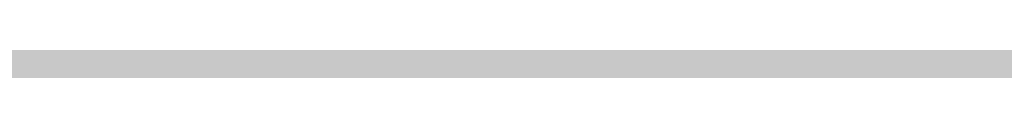
# Model space of a CAD drawing. Units: millimetres. Extents: x -22994 to 29398, y -19990 to 20176.
# Tile 97 of 135: x 229.428 to 230.597, y 84.571 to 84.585. Entities that reach past the tile are written whole.
import ezdxf
from ezdxf import colors
from ezdxf.entities.mleader import LeaderData, LeaderLine
from ezdxf.math import Vec2, Vec3

# ---------------------------------------------------------------- set-up
doc = ezdxf.new("R2010")
doc.units = ezdxf.units.MM
doc.header["$MEASUREMENT"] = 0
doc.layers.add('M-ANNO-TEXT', color=7, linetype='Continuous', lineweight=25)
doc.layers.add('M-DIMS', color=2, linetype='Continuous', lineweight=18)
doc.styles.get("Standard").update_dxf_attribs({"font": 'arial.ttf'})
doc.dimstyles.get("Standard").update_dxf_attribs({"dimtxt": 0.18, "dimasz": 10000, "dimexe": 0.18, "dimexo": 0.0625, "dimgap": 0.09, "dimtad": 0, "dimtih": 1, "dimtoh": 1, "dimdec": 0, "dimzin": 0, "dimdsep": 46, "dimtxsty": 'Standard', "dimcen": 0.09, "dimadec": 0, "dimazin": 0, "dimtfac": 1, "dimtdec": 0, "dimtofl": 0, "dimtmove": 0, "dimatfit": 3, "dimfxl": 1, "dimtolj": 1, "dimtzin": 0, "dimlwd": 30, "dimarcsym": 0})

# ---------------------------------------------------------------- blocks, each defined once
blk = doc.blocks.new('*D2')
at = {"layer": 'Defpoints', "color": 0, "transparency": 16777216}
for p in [(6.6773, 10.2713), (290.852, 10.2713), (290.852, -5.0787)]:
    blk.add_point(p, dxfattribs=at)
at = {"layer": 'M-DIMS', "color": 0, "lineweight": -2, "transparency": 16777216}
for p, q in [((6.6773, 10.2088), (6.6773, -5.2587)), ((290.852, 10.2088), (290.852, -5.2587))]:
    blk.add_line(p, q, dxfattribs=at)
at = {"layer": 'M-DIMS', "color": 0, "lineweight": 30, "transparency": 16777216}
for p, q in [((-9993.3227, -5.0787), (-19993.3227, -5.0787)), ((10290.852, -5.0787), (20290.852, -5.0787))]:
    blk.add_line(p, q, dxfattribs=at)
at = {"layer": 'M-DIMS', "color": 0, "transparency": 16777216}
for points in [[(-9993.3227, 1661.5879), (-9993.3227, -1671.7454), (6.6773, -5.0787)], [(10290.852, 1661.5879), (10290.852, -1671.7454), (290.852, -5.0787)]]:
    blk.add_solid(points, dxfattribs=at)
at = {"layer": 'M-DIMS', "color": 0, "transparency": 16777216, "insert": (148.7647, -5.0787), "char_height": 0.18, "attachment_point": 5}
blk.add_mtext('\\A1;284.2', dxfattribs=at)
blk = doc.blocks.new('*D3')
at = {"layer": 'Defpoints', "color": 0, "transparency": 16777216}
for p in [(110.2647, 204.1654), (110.2647, 176.3662), (95.8327, 127.967)]:
    blk.add_point(p, dxfattribs=at)
at = {"layer": 'M-DIMS', "color": 0, "lineweight": -2, "transparency": 16777216}
for p, q in [((95.8327, 128.0295), (95.8327, 204.3454)), ((110.2647, 176.4287), (110.2647, 204.3454))]:
    blk.add_line(p, q, dxfattribs=at)
at = {"layer": 'M-DIMS', "color": 0, "lineweight": 30, "transparency": 16777216}
for p, q in [((-9904.1673, 204.1654), (-19904.1673, 204.1654)), ((10110.2647, 204.1654), (20110.2647, 204.1654))]:
    blk.add_line(p, q, dxfattribs=at)
at = {"layer": 'M-DIMS', "color": 0, "transparency": 16777216}
for points in [[(-9904.1673, 1870.8321), (-9904.1673, -1462.5013), (95.8327, 204.1654)], [(10110.2647, 1870.8321), (10110.2647, -1462.5013), (110.2647, 204.1654)]]:
    blk.add_solid(points, dxfattribs=at)
at = {"layer": 'M-DIMS', "color": 0, "transparency": 16777216, "insert": (103.0487, 204.1654), "char_height": 0.18, "attachment_point": 5}
blk.add_mtext('\\A1;14.432', dxfattribs=at)
blk = doc.blocks.new('*D4')
at = {"layer": 'Defpoints', "color": 0, "transparency": 16777216}
for p in [(116.2647, 204.1654), (110.2647, 176.3662), (116.2647, 176.3662)]:
    blk.add_point(p, dxfattribs=at)
at = {"layer": 'M-DIMS', "color": 0, "lineweight": -2, "transparency": 16777216}
for p, q in [((110.2647, 176.4287), (110.2647, 204.3454)), ((116.2647, 176.4287), (116.2647, 204.3454))]:
    blk.add_line(p, q, dxfattribs=at)
at = {"layer": 'M-DIMS', "color": 0, "lineweight": 30, "transparency": 16777216}
for p, q in [((-9889.7353, 204.1654), (-19889.7353, 204.1654)), ((10116.2647, 204.1654), (20116.2647, 204.1654))]:
    blk.add_line(p, q, dxfattribs=at)
at = {"layer": 'M-DIMS', "color": 0, "transparency": 16777216}
for points in [[(-9889.7353, 1870.8321), (-9889.7353, -1462.5013), (110.2647, 204.1654)], [(10116.2647, 1870.8321), (10116.2647, -1462.5013), (116.2647, 204.1654)]]:
    blk.add_solid(points, dxfattribs=at)
at = {"layer": 'M-DIMS', "color": 0, "transparency": 16777216, "insert": (113.2647, 204.1654), "char_height": 0.18, "attachment_point": 5}
blk.add_mtext('\\A1;6', dxfattribs=at)
blk = doc.blocks.new('*D5')
at = {"layer": 'Defpoints', "color": 0, "transparency": 16777216}
for p in [(181.2647, 204.1654), (116.2647, 176.3662), (181.2647, 176.3662)]:
    blk.add_point(p, dxfattribs=at)
at = {"layer": 'M-DIMS', "color": 0, "lineweight": -2, "transparency": 16777216}
for p, q in [((116.2647, 176.4287), (116.2647, 204.3454)), ((181.2647, 176.4287), (181.2647, 204.3454))]:
    blk.add_line(p, q, dxfattribs=at)
at = {"layer": 'M-DIMS', "color": 0, "lineweight": 30, "transparency": 16777216}
for p, q in [((-9883.7353, 204.1654), (-19883.7353, 204.1654)), ((10181.2647, 204.1654), (20181.2647, 204.1654))]:
    blk.add_line(p, q, dxfattribs=at)
at = {"layer": 'M-DIMS', "color": 0, "transparency": 16777216}
for points in [[(-9883.7353, 1870.8321), (-9883.7353, -1462.5013), (116.2647, 204.1654)], [(10181.2647, 1870.8321), (10181.2647, -1462.5013), (181.2647, 204.1654)]]:
    blk.add_solid(points, dxfattribs=at)
at = {"layer": 'M-DIMS', "color": 0, "transparency": 16777216, "insert": (148.7647, 204.1654), "char_height": 0.18, "attachment_point": 5}
blk.add_mtext('\\A1;65', dxfattribs=at)
blk = doc.blocks.new('*D6')
at = {"layer": 'Defpoints', "color": 0, "transparency": 16777216}
for p in [(187.2647, 204.1654), (181.2647, 176.3662), (187.2647, 176.3662)]:
    blk.add_point(p, dxfattribs=at)
at = {"layer": 'M-DIMS', "color": 0, "lineweight": -2, "transparency": 16777216}
for p, q in [((181.2647, 176.4287), (181.2647, 204.3454)), ((187.2647, 176.4287), (187.2647, 204.3454))]:
    blk.add_line(p, q, dxfattribs=at)
at = {"layer": 'M-DIMS', "color": 0, "lineweight": 30, "transparency": 16777216}
for p, q in [((-9818.7353, 204.1654), (-19818.7353, 204.1654)), ((10187.2647, 204.1654), (20187.2647, 204.1654))]:
    blk.add_line(p, q, dxfattribs=at)
at = {"layer": 'M-DIMS', "color": 0, "transparency": 16777216}
for points in [[(-9818.7353, 1870.8321), (-9818.7353, -1462.5013), (181.2647, 204.1654)], [(10187.2647, 1870.8321), (10187.2647, -1462.5013), (187.2647, 204.1654)]]:
    blk.add_solid(points, dxfattribs=at)
at = {"layer": 'M-DIMS', "color": 0, "transparency": 16777216, "insert": (184.2647, 204.1654), "char_height": 0.18, "attachment_point": 5}
blk.add_mtext('\\A1;6', dxfattribs=at)
blk = doc.blocks.new('*D7')
at = {"layer": 'Defpoints', "color": 0, "transparency": 16777216}
for p in [(201.6967, 204.1654), (187.2647, 176.3662), (201.6967, 127.967)]:
    blk.add_point(p, dxfattribs=at)
at = {"layer": 'M-DIMS', "color": 0, "lineweight": -2, "transparency": 16777216}
for p, q in [((187.2647, 176.4287), (187.2647, 204.3454)), ((201.6967, 128.0295), (201.6967, 204.3454))]:
    blk.add_line(p, q, dxfattribs=at)
at = {"layer": 'M-DIMS', "color": 0, "lineweight": 30, "transparency": 16777216}
for p, q in [((-9812.7353, 204.1654), (-19812.7353, 204.1654)), ((10201.6967, 204.1654), (20201.6967, 204.1654))]:
    blk.add_line(p, q, dxfattribs=at)
at = {"layer": 'M-DIMS', "color": 0, "transparency": 16777216}
for points in [[(-9812.7353, 1870.8321), (-9812.7353, -1462.5013), (187.2647, 204.1654)], [(10201.6967, 1870.8321), (10201.6967, -1462.5013), (201.6967, 204.1654)]]:
    blk.add_solid(points, dxfattribs=at)
at = {"layer": 'M-DIMS', "color": 0, "transparency": 16777216, "insert": (194.4807, 204.1654), "char_height": 0.18, "attachment_point": 5}
blk.add_mtext('\\A1;14.432', dxfattribs=at)
blk = doc.blocks.new('*D8')
at = {"layer": 'Defpoints', "color": 0, "transparency": 16777216}
for p in [(227.6485, 204.1654), (227.6485, 146.7296), (201.6967, 127.967)]:
    blk.add_point(p, dxfattribs=at)
at = {"layer": 'M-DIMS', "color": 0, "lineweight": -2, "transparency": 16777216}
for p, q in [((201.6967, 128.0295), (201.6967, 204.3454)), ((227.6485, 146.7921), (227.6485, 204.3454))]:
    blk.add_line(p, q, dxfattribs=at)
at = {"layer": 'M-DIMS', "color": 0, "lineweight": 30, "transparency": 16777216}
for p, q in [((-9798.3033, 204.1654), (-19798.3033, 204.1654)), ((10227.6485, 204.1654), (20227.6485, 204.1654))]:
    blk.add_line(p, q, dxfattribs=at)
at = {"layer": 'M-DIMS', "color": 0, "transparency": 16777216}
for points in [[(-9798.3033, 1870.8321), (-9798.3033, -1462.5013), (201.6967, 204.1654)], [(10227.6485, 1870.8321), (10227.6485, -1462.5013), (227.6485, 204.1654)]]:
    blk.add_solid(points, dxfattribs=at)
at = {"layer": 'M-DIMS', "color": 0, "transparency": 16777216, "insert": (214.6726, 204.1654), "char_height": 0.18, "attachment_point": 5}
blk.add_mtext('\\A1;25.95', dxfattribs=at)
blk = doc.blocks.new('*D9')
at = {"layer": 'Defpoints', "color": 0, "transparency": 16777216}
for p in [(187.2647, 176.3662), (306.202, 176.3662), (290.852, 10.2713)]:
    blk.add_point(p, dxfattribs=at)
at = {"layer": 'M-DIMS', "color": 0, "lineweight": 30, "transparency": 16777216}
for p, q in [((306.202, 10176.3662), (306.202, 20176.3662)), ((306.202, -9989.7287), (306.202, -19989.7287))]:
    blk.add_line(p, q, dxfattribs=at)
at = {"layer": 'M-DIMS', "color": 0, "lineweight": -2, "transparency": 16777216}
for p, q in [((187.3272, 176.3662), (306.382, 176.3662)), ((290.9145, 10.2713), (306.382, 10.2713))]:
    blk.add_line(p, q, dxfattribs=at)
at = {"layer": 'M-DIMS', "color": 0, "transparency": 16777216}
for points in [[(-1360.4646, 10176.3662), (1972.8687, 10176.3662), (306.202, 176.3662)], [(-1360.4646, -9989.7287), (1972.8687, -9989.7287), (306.202, 10.2713)]]:
    blk.add_solid(points, dxfattribs=at)
at = {"layer": 'M-DIMS', "color": 0, "transparency": 16777216, "insert": (306.202, 93.3187), "char_height": 0.18, "attachment_point": 5}
blk.add_mtext('\\A1;166.1', dxfattribs=at)
blk = doc.blocks.new('*D10')
at = {"layer": 'Defpoints', "color": 0, "transparency": 16777216}
for p in [(125.6498, 136.0713), (133.3459, 136.0713), (133.3459, -5.0787)]:
    blk.add_point(p, dxfattribs=at)
at = {"layer": 'M-DIMS', "color": 0, "lineweight": -2, "transparency": 16777216}
for p, q in [((125.6498, 136.0088), (125.6498, -5.2587)), ((133.3459, 136.0088), (133.3459, -5.2587))]:
    blk.add_line(p, q, dxfattribs=at)
at = {"layer": 'M-DIMS', "color": 0, "lineweight": 30, "transparency": 16777216}
for p, q in [((-9874.3502, -5.0787), (-19874.3502, -5.0787)), ((10133.3459, -5.0787), (20133.3459, -5.0787))]:
    blk.add_line(p, q, dxfattribs=at)
at = {"layer": 'M-DIMS', "color": 0, "transparency": 16777216}
for points in [[(-9874.3502, 1661.5879), (-9874.3502, -1671.7454), (125.6498, -5.0787)], [(10133.3459, 1661.5879), (10133.3459, -1671.7454), (133.3459, -5.0787)]]:
    blk.add_solid(points, dxfattribs=at)
at = {"layer": 'M-DIMS', "color": 0, "transparency": 16777216, "insert": (129.4978, -5.0787), "char_height": 0.18, "attachment_point": 5}
blk.add_mtext('\\A1;7.696', dxfattribs=at)
blk = doc.blocks.new('*D11')
at = {"layer": 'Defpoints', "color": 0, "transparency": 16777216}
for p in [(133.3459, 136.0713), (135.6498, 136.0713), (135.6498, -5.0787)]:
    blk.add_point(p, dxfattribs=at)
at = {"layer": 'M-DIMS', "color": 0, "lineweight": -2, "transparency": 16777216}
for p, q in [((133.3459, 136.0088), (133.3459, -5.2587)), ((135.6498, 136.0088), (135.6498, -5.2587))]:
    blk.add_line(p, q, dxfattribs=at)
at = {"layer": 'M-DIMS', "color": 0, "lineweight": 30, "transparency": 16777216}
for p, q in [((-9866.6541, -5.0787), (-19866.6541, -5.0787)), ((10135.6498, -5.0787), (20135.6498, -5.0787))]:
    blk.add_line(p, q, dxfattribs=at)
at = {"layer": 'M-DIMS', "color": 0, "transparency": 16777216}
for points in [[(-9866.6541, 1661.5879), (-9866.6541, -1671.7454), (133.3459, -5.0787)], [(10135.6498, 1661.5879), (10135.6498, -1671.7454), (135.6498, -5.0787)]]:
    blk.add_solid(points, dxfattribs=at)
at = {"layer": 'M-DIMS', "color": 0, "transparency": 16777216, "insert": (134.4978, -5.0787), "char_height": 0.18, "attachment_point": 5}
blk.add_mtext('\\A1;2.304', dxfattribs=at)
blk = doc.blocks.new('*D12')
at = {"layer": 'Defpoints', "color": 0, "transparency": 16777216}
for p in [(135.6498, 136.0713), (145.6498, 136.0713), (145.6498, -5.0787)]:
    blk.add_point(p, dxfattribs=at)
at = {"layer": 'M-DIMS', "color": 0, "lineweight": -2, "transparency": 16777216}
for p, q in [((135.6498, 136.0088), (135.6498, -5.2587)), ((145.6498, 136.0088), (145.6498, -5.2587))]:
    blk.add_line(p, q, dxfattribs=at)
at = {"layer": 'M-DIMS', "color": 0, "lineweight": 30, "transparency": 16777216}
for p, q in [((-9864.3502, -5.0787), (-19864.3502, -5.0787)), ((10145.6498, -5.0787), (20145.6498, -5.0787))]:
    blk.add_line(p, q, dxfattribs=at)
at = {"layer": 'M-DIMS', "color": 0, "transparency": 16777216}
for points in [[(-9864.3502, 1661.5879), (-9864.3502, -1671.7454), (135.6498, -5.0787)], [(10145.6498, 1661.5879), (10145.6498, -1671.7454), (145.6498, -5.0787)]]:
    blk.add_solid(points, dxfattribs=at)
at = {"layer": 'M-DIMS', "color": 0, "transparency": 16777216, "insert": (140.6498, -5.0787), "char_height": 0.18, "attachment_point": 5}
blk.add_mtext('\\A1;10', dxfattribs=at)
blk = doc.blocks.new('*D13')
at = {"layer": 'Defpoints', "color": 0, "transparency": 16777216}
for p in [(145.6498, 136.0713), (155.6498, 136.0713), (155.6498, -5.0787)]:
    blk.add_point(p, dxfattribs=at)
at = {"layer": 'M-DIMS', "color": 0, "lineweight": -2, "transparency": 16777216}
for p, q in [((145.6498, 136.0088), (145.6498, -5.2587)), ((155.6498, 136.0088), (155.6498, -5.2587))]:
    blk.add_line(p, q, dxfattribs=at)
at = {"layer": 'M-DIMS', "color": 0, "lineweight": 30, "transparency": 16777216}
for p, q in [((-9854.3502, -5.0787), (-19854.3502, -5.0787)), ((10155.6498, -5.0787), (20155.6498, -5.0787))]:
    blk.add_line(p, q, dxfattribs=at)
at = {"layer": 'M-DIMS', "color": 0, "transparency": 16777216}
for points in [[(-9854.3502, 1661.5879), (-9854.3502, -1671.7454), (145.6498, -5.0787)], [(10155.6498, 1661.5879), (10155.6498, -1671.7454), (155.6498, -5.0787)]]:
    blk.add_solid(points, dxfattribs=at)
at = {"layer": 'M-DIMS', "color": 0, "transparency": 16777216, "insert": (150.6498, -5.0787), "char_height": 0.18, "attachment_point": 5}
blk.add_mtext('\\A1;10', dxfattribs=at)
blk = doc.blocks.new('*D14')
at = {"layer": 'Defpoints', "color": 0, "transparency": 16777216}
for p in [(155.6498, 136.0713), (165.6498, 136.0713), (165.6498, -5.0787)]:
    blk.add_point(p, dxfattribs=at)
at = {"layer": 'M-DIMS', "color": 0, "lineweight": -2, "transparency": 16777216}
for p, q in [((155.6498, 136.0088), (155.6498, -5.2587)), ((165.6498, 136.0088), (165.6498, -5.2587))]:
    blk.add_line(p, q, dxfattribs=at)
at = {"layer": 'M-DIMS', "color": 0, "lineweight": 30, "transparency": 16777216}
for p, q in [((-9844.3502, -5.0787), (-19844.3502, -5.0787)), ((10165.6498, -5.0787), (20165.6498, -5.0787))]:
    blk.add_line(p, q, dxfattribs=at)
at = {"layer": 'M-DIMS', "color": 0, "transparency": 16777216}
for points in [[(-9844.3502, 1661.5879), (-9844.3502, -1671.7454), (155.6498, -5.0787)], [(10165.6498, 1661.5879), (10165.6498, -1671.7454), (165.6498, -5.0787)]]:
    blk.add_solid(points, dxfattribs=at)
at = {"layer": 'M-DIMS', "color": 0, "transparency": 16777216, "insert": (160.6498, -5.0787), "char_height": 0.18, "attachment_point": 5}
blk.add_mtext('\\A1;10', dxfattribs=at)
blk = doc.blocks.new('*D15')
at = {"layer": 'Defpoints', "color": 0, "transparency": 16777216}
for p in [(173.3459, 154.788), (173.3459, 136.0713), (306.202, 136.0713)]:
    blk.add_point(p, dxfattribs=at)
at = {"layer": 'M-DIMS', "color": 0, "lineweight": 30, "transparency": 16777216}
for p, q in [((306.202, 10154.788), (306.202, 20154.788)), ((306.202, -9863.9287), (306.202, -19863.9287))]:
    blk.add_line(p, q, dxfattribs=at)
at = {"layer": 'M-DIMS', "color": 0, "lineweight": -2, "transparency": 16777216}
for p, q in [((173.4084, 154.788), (306.382, 154.788)), ((173.4084, 136.0713), (306.382, 136.0713))]:
    blk.add_line(p, q, dxfattribs=at)
at = {"layer": 'M-DIMS', "color": 0, "transparency": 16777216}
for points in [[(-1360.4646, 10154.788), (1972.8687, 10154.788), (306.202, 154.788)], [(-1360.4646, -9863.9287), (1972.8687, -9863.9287), (306.202, 136.0713)]]:
    blk.add_solid(points, dxfattribs=at)
at = {"layer": 'M-DIMS', "color": 0, "transparency": 16777216, "insert": (306.202, 145.4297), "char_height": 0.18, "attachment_point": 5}
blk.add_mtext('\\A1;18.717', dxfattribs=at)
blk = doc.blocks.new('*D16')
at = {"layer": 'Defpoints', "color": 0, "transparency": 16777216}
for p in [(120.1702, 204.1654), (110.4658, 48.0349), (120.1702, 48.0349)]:
    blk.add_point(p, dxfattribs=at)
at = {"layer": 'M-DIMS', "color": 0, "lineweight": -2, "transparency": 16777216}
for p, q in [((110.4658, 48.0974), (110.4658, 204.3454)), ((120.1702, 48.0974), (120.1702, 204.3454))]:
    blk.add_line(p, q, dxfattribs=at)
at = {"layer": 'M-DIMS', "color": 0, "lineweight": 30, "transparency": 16777216}
for p, q in [((-9889.5342, 204.1654), (-19889.5342, 204.1654)), ((10120.1702, 204.1654), (20120.1702, 204.1654))]:
    blk.add_line(p, q, dxfattribs=at)
at = {"layer": 'M-DIMS', "color": 0, "transparency": 16777216}
for points in [[(-9889.5342, 1870.8321), (-9889.5342, -1462.5013), (110.4658, 204.1654)], [(10120.1702, 1870.8321), (10120.1702, -1462.5013), (120.1702, 204.1654)]]:
    blk.add_solid(points, dxfattribs=at)
at = {"layer": 'M-DIMS', "color": 0, "transparency": 16777216, "insert": (115.318, 204.1654), "char_height": 0.18, "attachment_point": 5}
blk.add_mtext('\\A1;9.704', dxfattribs=at)
blk = doc.blocks.new('*D17')
at = {"layer": 'Defpoints', "color": 0, "transparency": 16777216}
for p in [(126.1702, 204.1654), (120.1702, 48.0349), (126.1702, 48.0349)]:
    blk.add_point(p, dxfattribs=at)
at = {"layer": 'M-DIMS', "color": 0, "lineweight": -2, "transparency": 16777216}
for p, q in [((120.1702, 48.0974), (120.1702, 204.3454)), ((126.1702, 48.0974), (126.1702, 204.3454))]:
    blk.add_line(p, q, dxfattribs=at)
at = {"layer": 'M-DIMS', "color": 0, "lineweight": 30, "transparency": 16777216}
for p, q in [((-9879.8298, 204.1654), (-19879.8298, 204.1654)), ((10126.1702, 204.1654), (20126.1702, 204.1654))]:
    blk.add_line(p, q, dxfattribs=at)
at = {"layer": 'M-DIMS', "color": 0, "transparency": 16777216}
for points in [[(-9879.8298, 1870.8321), (-9879.8298, -1462.5013), (120.1702, 204.1654)], [(10126.1702, 1870.8321), (10126.1702, -1462.5013), (126.1702, 204.1654)]]:
    blk.add_solid(points, dxfattribs=at)
at = {"layer": 'M-DIMS', "color": 0, "transparency": 16777216, "insert": (123.1702, 204.1654), "char_height": 0.18, "attachment_point": 5}
blk.add_mtext('\\A1;6', dxfattribs=at)
blk = doc.blocks.new('*D18')
at = {"layer": 'Defpoints', "color": 0, "transparency": 16777216}
for p in [(132.1702, 204.1654), (126.1702, 48.0349), (132.1702, 48.0349)]:
    blk.add_point(p, dxfattribs=at)
at = {"layer": 'M-DIMS', "color": 0, "lineweight": -2, "transparency": 16777216}
for p, q in [((126.1702, 48.0974), (126.1702, 204.3454)), ((132.1702, 48.0974), (132.1702, 204.3454))]:
    blk.add_line(p, q, dxfattribs=at)
at = {"layer": 'M-DIMS', "color": 0, "lineweight": 30, "transparency": 16777216}
for p, q in [((-9873.8298, 204.1654), (-19873.8298, 204.1654)), ((10132.1702, 204.1654), (20132.1702, 204.1654))]:
    blk.add_line(p, q, dxfattribs=at)
at = {"layer": 'M-DIMS', "color": 0, "transparency": 16777216}
for points in [[(-9873.8298, 1870.8321), (-9873.8298, -1462.5013), (126.1702, 204.1654)], [(10132.1702, 1870.8321), (10132.1702, -1462.5013), (132.1702, 204.1654)]]:
    blk.add_solid(points, dxfattribs=at)
at = {"layer": 'M-DIMS', "color": 0, "transparency": 16777216, "insert": (129.1702, 204.1654), "char_height": 0.18, "attachment_point": 5}
blk.add_mtext('\\A1;6', dxfattribs=at)
blk = doc.blocks.new('*D19')
at = {"layer": 'Defpoints', "color": 0, "transparency": 16777216}
for p in [(138.1702, 204.1654), (132.1702, 48.0349), (138.1702, 48.0349)]:
    blk.add_point(p, dxfattribs=at)
at = {"layer": 'M-DIMS', "color": 0, "lineweight": -2, "transparency": 16777216}
for p, q in [((132.1702, 48.0974), (132.1702, 204.3454)), ((138.1702, 48.0974), (138.1702, 204.3454))]:
    blk.add_line(p, q, dxfattribs=at)
at = {"layer": 'M-DIMS', "color": 0, "lineweight": 30, "transparency": 16777216}
for p, q in [((-9867.8298, 204.1654), (-19867.8298, 204.1654)), ((10138.1702, 204.1654), (20138.1702, 204.1654))]:
    blk.add_line(p, q, dxfattribs=at)
at = {"layer": 'M-DIMS', "color": 0, "transparency": 16777216}
for points in [[(-9867.8298, 1870.8321), (-9867.8298, -1462.5013), (132.1702, 204.1654)], [(10138.1702, 1870.8321), (10138.1702, -1462.5013), (138.1702, 204.1654)]]:
    blk.add_solid(points, dxfattribs=at)
at = {"layer": 'M-DIMS', "color": 0, "transparency": 16777216, "insert": (135.1702, 204.1654), "char_height": 0.18, "attachment_point": 5}
blk.add_mtext('\\A1;6', dxfattribs=at)
blk = doc.blocks.new('*D20')
at = {"layer": 'Defpoints', "color": 0, "transparency": 16777216}
for p in [(144.1702, 204.1654), (138.1702, 48.0349), (144.1702, 48.0349)]:
    blk.add_point(p, dxfattribs=at)
at = {"layer": 'M-DIMS', "color": 0, "lineweight": -2, "transparency": 16777216}
for p, q in [((138.1702, 48.0974), (138.1702, 204.3454)), ((144.1702, 48.0974), (144.1702, 204.3454))]:
    blk.add_line(p, q, dxfattribs=at)
at = {"layer": 'M-DIMS', "color": 0, "lineweight": 30, "transparency": 16777216}
for p, q in [((-9861.8298, 204.1654), (-19861.8298, 204.1654)), ((10144.1702, 204.1654), (20144.1702, 204.1654))]:
    blk.add_line(p, q, dxfattribs=at)
at = {"layer": 'M-DIMS', "color": 0, "transparency": 16777216}
for points in [[(-9861.8298, 1870.8321), (-9861.8298, -1462.5013), (138.1702, 204.1654)], [(10144.1702, 1870.8321), (10144.1702, -1462.5013), (144.1702, 204.1654)]]:
    blk.add_solid(points, dxfattribs=at)
at = {"layer": 'M-DIMS', "color": 0, "transparency": 16777216, "insert": (141.1702, 204.1654), "char_height": 0.18, "attachment_point": 5}
blk.add_mtext('\\A1;6', dxfattribs=at)
blk = doc.blocks.new('*D21')
at = {"layer": 'Defpoints', "color": 0, "transparency": 16777216}
for p in [(149.1157, 204.1654), (144.1702, 48.0349), (149.1157, 48.0349)]:
    blk.add_point(p, dxfattribs=at)
at = {"layer": 'M-DIMS', "color": 0, "lineweight": -2, "transparency": 16777216}
for p, q in [((144.1702, 48.0974), (144.1702, 204.3454)), ((149.1157, 48.0974), (149.1157, 204.3454))]:
    blk.add_line(p, q, dxfattribs=at)
at = {"layer": 'M-DIMS', "color": 0, "lineweight": 30, "transparency": 16777216}
for p, q in [((-9855.8298, 204.1654), (-19855.8298, 204.1654)), ((10149.1157, 204.1654), (20149.1157, 204.1654))]:
    blk.add_line(p, q, dxfattribs=at)
at = {"layer": 'M-DIMS', "color": 0, "transparency": 16777216}
for points in [[(-9855.8298, 1870.8321), (-9855.8298, -1462.5013), (144.1702, 204.1654)], [(10149.1157, 1870.8321), (10149.1157, -1462.5013), (149.1157, 204.1654)]]:
    blk.add_solid(points, dxfattribs=at)
at = {"layer": 'M-DIMS', "color": 0, "transparency": 16777216, "insert": (146.6429, 204.1654), "char_height": 0.18, "attachment_point": 5}
blk.add_mtext('\\A1;4.945', dxfattribs=at)
blk = doc.blocks.new('*D22')
at = {"layer": 'Defpoints', "color": 0, "transparency": 16777216}
for p in [(149.1157, 30.9895), (155.1157, 30.9895), (155.1157, -5.0787)]:
    blk.add_point(p, dxfattribs=at)
at = {"layer": 'M-DIMS', "color": 0, "lineweight": -2, "transparency": 16777216}
for p, q in [((149.1157, 30.927), (149.1157, -5.2587)), ((155.1157, 30.927), (155.1157, -5.2587))]:
    blk.add_line(p, q, dxfattribs=at)
at = {"layer": 'M-DIMS', "color": 0, "lineweight": 30, "transparency": 16777216}
for p, q in [((-9850.8843, -5.0787), (-19850.8843, -5.0787)), ((10155.1157, -5.0787), (20155.1157, -5.0787))]:
    blk.add_line(p, q, dxfattribs=at)
at = {"layer": 'M-DIMS', "color": 0, "transparency": 16777216}
for points in [[(-9850.8843, 1661.5879), (-9850.8843, -1671.7454), (149.1157, -5.0787)], [(10155.1157, 1661.5879), (10155.1157, -1671.7454), (155.1157, -5.0787)]]:
    blk.add_solid(points, dxfattribs=at)
at = {"layer": 'M-DIMS', "color": 0, "transparency": 16777216, "insert": (152.1157, -5.0787), "char_height": 0.18, "attachment_point": 5}
blk.add_mtext('\\A1;6', dxfattribs=at)
blk = doc.blocks.new('*D23')
at = {"layer": 'Defpoints', "color": 0, "transparency": 16777216}
for p in [(155.1157, 30.9895), (161.1157, 30.9895), (161.1157, -5.0787)]:
    blk.add_point(p, dxfattribs=at)
at = {"layer": 'M-DIMS', "color": 0, "lineweight": -2, "transparency": 16777216}
for p, q in [((155.1157, 30.927), (155.1157, -5.2587)), ((161.1157, 30.927), (161.1157, -5.2587))]:
    blk.add_line(p, q, dxfattribs=at)
at = {"layer": 'M-DIMS', "color": 0, "lineweight": 30, "transparency": 16777216}
for p, q in [((-9844.8843, -5.0787), (-19844.8843, -5.0787)), ((10161.1157, -5.0787), (20161.1157, -5.0787))]:
    blk.add_line(p, q, dxfattribs=at)
at = {"layer": 'M-DIMS', "color": 0, "transparency": 16777216}
for points in [[(-9844.8843, 1661.5879), (-9844.8843, -1671.7454), (155.1157, -5.0787)], [(10161.1157, 1661.5879), (10161.1157, -1671.7454), (161.1157, -5.0787)]]:
    blk.add_solid(points, dxfattribs=at)
at = {"layer": 'M-DIMS', "color": 0, "transparency": 16777216, "insert": (158.1157, -5.0787), "char_height": 0.18, "attachment_point": 5}
blk.add_mtext('\\A1;6', dxfattribs=at)
blk = doc.blocks.new('*D24')
at = {"layer": 'Defpoints', "color": 0, "transparency": 16777216}
for p in [(161.1157, 30.9895), (166.4387, 30.9895), (166.4387, -5.0787)]:
    blk.add_point(p, dxfattribs=at)
at = {"layer": 'M-DIMS', "color": 0, "lineweight": -2, "transparency": 16777216}
for p, q in [((161.1157, 30.927), (161.1157, -5.2587)), ((166.4387, 30.927), (166.4387, -5.2587))]:
    blk.add_line(p, q, dxfattribs=at)
at = {"layer": 'M-DIMS', "color": 0, "lineweight": 30, "transparency": 16777216}
for p, q in [((-9838.8843, -5.0787), (-19838.8843, -5.0787)), ((10166.4387, -5.0787), (20166.4387, -5.0787))]:
    blk.add_line(p, q, dxfattribs=at)
at = {"layer": 'M-DIMS', "color": 0, "transparency": 16777216}
for points in [[(-9838.8843, 1661.5879), (-9838.8843, -1671.7454), (161.1157, -5.0787)], [(10166.4387, 1661.5879), (10166.4387, -1671.7454), (166.4387, -5.0787)]]:
    blk.add_solid(points, dxfattribs=at)
at = {"layer": 'M-DIMS', "color": 0, "transparency": 16777216, "insert": (163.7772, -5.0787), "char_height": 0.18, "attachment_point": 5}
blk.add_mtext('\\A1;5.323', dxfattribs=at)
blk = doc.blocks.new('*D25')
at = {"layer": 'Defpoints', "color": 0, "transparency": 16777216}
for p in [(166.4387, 30.9895), (172.4387, 30.9895), (172.4387, -5.0787)]:
    blk.add_point(p, dxfattribs=at)
at = {"layer": 'M-DIMS', "color": 0, "lineweight": -2, "transparency": 16777216}
for p, q in [((166.4387, 30.927), (166.4387, -5.2587)), ((172.4387, 30.927), (172.4387, -5.2587))]:
    blk.add_line(p, q, dxfattribs=at)
at = {"layer": 'M-DIMS', "color": 0, "lineweight": 30, "transparency": 16777216}
for p, q in [((-9833.5613, -5.0787), (-19833.5613, -5.0787)), ((10172.4387, -5.0787), (20172.4387, -5.0787))]:
    blk.add_line(p, q, dxfattribs=at)
at = {"layer": 'M-DIMS', "color": 0, "transparency": 16777216}
for points in [[(-9833.5613, 1661.5879), (-9833.5613, -1671.7454), (166.4387, -5.0787)], [(10172.4387, 1661.5879), (10172.4387, -1671.7454), (172.4387, -5.0787)]]:
    blk.add_solid(points, dxfattribs=at)
at = {"layer": 'M-DIMS', "color": 0, "transparency": 16777216, "insert": (169.4387, -5.0787), "char_height": 0.18, "attachment_point": 5}
blk.add_mtext('\\A1;6', dxfattribs=at)
blk = doc.blocks.new('*D26')
at = {"layer": 'Defpoints', "color": 0, "transparency": 16777216}
for p in [(172.4387, 30.9895), (178.4387, 30.9895), (178.4387, -5.0787)]:
    blk.add_point(p, dxfattribs=at)
at = {"layer": 'M-DIMS', "color": 0, "lineweight": -2, "transparency": 16777216}
for p, q in [((172.4387, 30.927), (172.4387, -5.2587)), ((178.4387, 30.927), (178.4387, -5.2587))]:
    blk.add_line(p, q, dxfattribs=at)
at = {"layer": 'M-DIMS', "color": 0, "lineweight": 30, "transparency": 16777216}
for p, q in [((-9827.5613, -5.0787), (-19827.5613, -5.0787)), ((10178.4387, -5.0787), (20178.4387, -5.0787))]:
    blk.add_line(p, q, dxfattribs=at)
at = {"layer": 'M-DIMS', "color": 0, "transparency": 16777216}
for points in [[(-9827.5613, 1661.5879), (-9827.5613, -1671.7454), (172.4387, -5.0787)], [(10178.4387, 1661.5879), (10178.4387, -1671.7454), (178.4387, -5.0787)]]:
    blk.add_solid(points, dxfattribs=at)
at = {"layer": 'M-DIMS', "color": 0, "transparency": 16777216, "insert": (175.4387, -5.0787), "char_height": 0.18, "attachment_point": 5}
blk.add_mtext('\\A1;6', dxfattribs=at)
blk = doc.blocks.new('*D27')
at = {"layer": 'Defpoints', "color": 0, "transparency": 16777216}
for p in [(178.4387, 30.9895), (188.1175, 30.9895), (188.1175, -5.0787)]:
    blk.add_point(p, dxfattribs=at)
at = {"layer": 'M-DIMS', "color": 0, "lineweight": -2, "transparency": 16777216}
for p, q in [((178.4387, 30.927), (178.4387, -5.2587)), ((188.1175, 30.927), (188.1175, -5.2587))]:
    blk.add_line(p, q, dxfattribs=at)
at = {"layer": 'M-DIMS', "color": 0, "lineweight": 30, "transparency": 16777216}
for p, q in [((-9821.5613, -5.0787), (-19821.5613, -5.0787)), ((10188.1175, -5.0787), (20188.1175, -5.0787))]:
    blk.add_line(p, q, dxfattribs=at)
at = {"layer": 'M-DIMS', "color": 0, "transparency": 16777216}
for points in [[(-9821.5613, 1661.5879), (-9821.5613, -1671.7454), (178.4387, -5.0787)], [(10188.1175, 1661.5879), (10188.1175, -1671.7454), (188.1175, -5.0787)]]:
    blk.add_solid(points, dxfattribs=at)
at = {"layer": 'M-DIMS', "color": 0, "transparency": 16777216, "insert": (183.2781, -5.0787), "char_height": 0.18, "attachment_point": 5}
blk.add_mtext('\\A1;9.679', dxfattribs=at)
blk = doc.blocks.new('*D28')
at = {"layer": 'Defpoints', "color": 0, "transparency": 16777216}
for p in [(188.1175, 48.0349), (306.202, 48.0349), (188.1175, 30.9895)]:
    blk.add_point(p, dxfattribs=at)
at = {"layer": 'M-DIMS', "color": 0, "lineweight": 30, "transparency": 16777216}
for p, q in [((306.202, 10048.0349), (306.202, 20048.0349)), ((306.202, -9969.0105), (306.202, -19969.0105))]:
    blk.add_line(p, q, dxfattribs=at)
at = {"layer": 'M-DIMS', "color": 0, "lineweight": -2, "transparency": 16777216}
for p, q in [((188.18, 48.0349), (306.382, 48.0349)), ((188.18, 30.9895), (306.382, 30.9895))]:
    blk.add_line(p, q, dxfattribs=at)
at = {"layer": 'M-DIMS', "color": 0, "transparency": 16777216}
for points in [[(-1360.4646, 10048.0349), (1972.8687, 10048.0349), (306.202, 48.0349)], [(-1360.4646, -9969.0105), (1972.8687, -9969.0105), (306.202, 30.9895)]]:
    blk.add_solid(points, dxfattribs=at)
at = {"layer": 'M-DIMS', "color": 0, "transparency": 16777216, "insert": (306.202, 39.5122), "char_height": 0.18, "attachment_point": 5}
blk.add_mtext('\\A1;17.045', dxfattribs=at)
blk = doc.blocks.new('*D29')
at = {"layer": 'Defpoints', "color": 0, "transparency": 16777216}
for p in [(36.8006, 80.045), (64.0296, 80.045)]:
    blk.add_point(p, dxfattribs=at)
at = {"layer": 'M-DIMS', "color": 0, "lineweight": -2, "transparency": 16777216}
for p, q in [((50.4151, 79.955), (50.4151, 80.135)), ((50.3251, 80.045), (50.5051, 80.045))]:
    blk.add_line(p, q, dxfattribs=at)
at = {"layer": 'M-DIMS', "color": 0, "lineweight": 30, "transparency": 16777216}
blk.add_line((20064.0296, 80.0303), (10064.0296, 80.0377), dxfattribs=at)
at = {"layer": 'M-DIMS', "color": 0, "transparency": 16777216}
blk.add_solid([(10064.0309, 1746.7043), (10064.0284, -1586.629), (64.0296, 80.045)], dxfattribs=at)
at = {"layer": 'M-DIMS', "color": 0, "transparency": 16777216, "insert": (20064.5213, 80.0303), "char_height": 0.18, "attachment_point": 5}
blk.add_mtext('\\A1;∅27.23', dxfattribs=at)
blk = doc.blocks.new('*D30')
at = {"layer": 'Defpoints', "color": 0, "transparency": 16777216}
for p in [(216.3148, 146.7291), (238.9821, 146.73)]:
    blk.add_point(p, dxfattribs=at)
at = {"layer": 'M-DIMS', "color": 0, "lineweight": 30, "transparency": 16777216}
blk.add_line((20238.9821, 147.4959), (10238.9821, 147.1129), dxfattribs=at)
at = {"layer": 'M-DIMS', "color": 0, "lineweight": -2, "transparency": 16777216}
for p, q in [((227.6485, 146.6396), (227.6485, 146.8196)), ((227.5585, 146.7296), (227.7385, 146.7296))]:
    blk.add_line(p, q, dxfattribs=at)
at = {"layer": 'M-DIMS', "color": 0, "transparency": 16777216}
blk.add_solid([(10238.9183, 1813.7796), (10239.0459, -1519.5537), (238.9821, 146.73)], dxfattribs=at)
at = {"layer": 'M-DIMS', "color": 0, "transparency": 16777216, "insert": (20239.5436, 147.4959), "char_height": 0.18, "attachment_point": 5}
blk.add_mtext('\\A1;∅22.667', dxfattribs=at)
blk = doc.blocks.new('*D31')
at = {"layer": 'Defpoints', "color": 0, "transparency": 16777216}
for p in [(223.1641, 146.7291), (232.1328, 146.73)]:
    blk.add_point(p, dxfattribs=at)
at = {"layer": 'M-DIMS', "color": 0, "lineweight": 30, "transparency": 16777216}
blk.add_line((20232.1327, 148.6656), (10232.1328, 147.6978), dxfattribs=at)
at = {"layer": 'M-DIMS', "color": 0, "lineweight": -2, "transparency": 16777216}
for p, q in [((227.6485, 146.6396), (227.6485, 146.8196)), ((227.5585, 146.7296), (227.7385, 146.7296))]:
    blk.add_line(p, q, dxfattribs=at)
at = {"layer": 'M-DIMS', "color": 0, "transparency": 16777216}
blk.add_solid([(10231.9715, 1814.3645), (10232.2941, -1518.9688), (232.1328, 146.73)], dxfattribs=at)
at = {"layer": 'M-DIMS', "color": 0, "transparency": 16777216, "insert": (20232.6245, 148.6656), "char_height": 0.18, "attachment_point": 5}
blk.add_mtext('\\A1;∅8.969', dxfattribs=at)
blk = doc.blocks.new('*D33')
at = {"layer": 'Defpoints', "color": 0, "transparency": 16777216}
for p in [(229.5613, 154.3773), (232.9972, 153.3509)]:
    blk.add_point(p, dxfattribs=at)
at = {"layer": 'M-DIMS', "color": 0, "lineweight": -2, "transparency": 16777216}
for p, q in [((229.5613, 154.2873), (229.5613, 154.4673)), ((229.4713, 154.3773), (229.6513, 154.3773))]:
    blk.add_line(p, q, dxfattribs=at)
at = {"layer": 'M-DIMS', "color": 0, "lineweight": 30, "transparency": 16777216}
for p, q in [((19396.3388, -5570.8378), (9814.668, -2708.7434)), ((29396.3388, -5570.8378), (19396.3388, -5570.8378))]:
    blk.add_line(p, q, dxfattribs=at)
at = {"layer": 'M-DIMS', "color": 0, "transparency": 16777216}
blk.add_solid([(10291.6837, -1111.7983), (9337.6523, -4305.6886), (232.9972, 153.3509)], dxfattribs=at)
at = {"layer": 'M-DIMS', "color": 0, "transparency": 16777216, "insert": (29397.0125, -5570.8378), "char_height": 0.18, "attachment_point": 5}
blk.add_mtext('\\A1;6X R3.586', dxfattribs=at)
blk = doc.blocks.new('*D36')
at = {"layer": 'Defpoints', "color": 0, "transparency": 16777216}
for p in [(46.39, 31.3035), (46.3875, 26.5934)]:
    blk.add_point(p, dxfattribs=at)
at = {"layer": 'M-DIMS', "color": 0, "lineweight": 30, "transparency": 16777216}
for p, q in [((57.1499, 20031.3006), (51.77, 10031.302)), ((10057.1499, 20031.3006), (57.1499, 20031.3006))]:
    blk.add_line(p, q, dxfattribs=at)
at = {"layer": 'M-DIMS', "color": 0, "lineweight": -2, "transparency": 16777216}
for p, q in [((46.3887, 28.8585), (46.3887, 29.0385)), ((46.2987, 28.9485), (46.4787, 28.9485))]:
    blk.add_line(p, q, dxfattribs=at)
at = {"layer": 'M-DIMS', "color": 0, "transparency": 16777216}
blk.add_solid([(-1614.8965, 10032.1987), (1718.4364, 10030.4054), (46.39, 31.3035)], dxfattribs=at)
at = {"layer": 'M-DIMS', "color": 0, "transparency": 16777216, "insert": (10057.5542, 20031.3006), "char_height": 0.18, "attachment_point": 5}
blk.add_mtext('\\A1;∅4.71', dxfattribs=at)
blk = doc.blocks.new('*D37')
at = {"layer": 'Defpoints', "color": 0, "transparency": 16777216}
for p in [(54.8343, 118.6145), (59.4936, 118.614)]:
    blk.add_point(p, dxfattribs=at)
at = {"layer": 'M-DIMS', "color": 0, "lineweight": -2, "transparency": 16777216}
for p, q in [((57.1639, 118.5243), (57.1639, 118.7043)), ((57.0739, 118.6143), (57.2539, 118.6143))]:
    blk.add_line(p, q, dxfattribs=at)
at = {"layer": 'M-DIMS', "color": 0, "lineweight": 30, "transparency": 16777216}
blk.add_line((20059.4934, 116.2531), (10059.4935, 117.4336), dxfattribs=at)
at = {"layer": 'M-DIMS', "color": 0, "transparency": 16777216}
blk.add_solid([(10059.6902, 1784.1002), (10059.2968, -1549.2331), (59.4936, 118.614)], dxfattribs=at)
at = {"layer": 'M-DIMS', "color": 0, "transparency": 16777216, "insert": (20059.9852, 116.2531), "char_height": 0.18, "attachment_point": 5}
blk.add_mtext('\\A1;∅4.659', dxfattribs=at)

msp = doc.modelspace()

# ---------------------------------------------------------------- dimensions: what is measured, and where the dimension line sits
at = {"layer": 'M-DIMS'}
for base, p1, p2, override, picture, middle in [((306.202, 176.3662), (290.852, 10.2713), (187.2647, 176.3662), {"dimdec": 1, "dimlfac": 1, "dimrnd": 0, "dimzin": 0, "dimdsep": 46, "dimlunit": 2}, '*D9', (306.202, 93.3187)), ((306.202, 136.0713), (173.3459, 154.788), (173.3459, 136.0713), {"dimdec": 3, "dimlfac": 1, "dimrnd": 0, "dimzin": 0, "dimdsep": 46, "dimlunit": 2}, '*D15', (306.202, 145.4297)), ((306.202, 48.0349), (188.1175, 30.9895), (188.1175, 48.0349), {"dimdec": 3, "dimlfac": 1, "dimrnd": 0, "dimzin": 0, "dimdsep": 46, "dimlunit": 2}, '*D28', (306.202, 39.5122))]:
    dim = msp.add_linear_dim(base=base, p1=p1, p2=p2, angle=90, dimstyle='Standard', override=override, dxfattribs=at)
    dim.commit()
    dim.dimension.update_dxf_attribs({"geometry": picture, "text_midpoint": middle})
for p1, p2, override, picture, middle in [((46.3875, 26.5934), (46.39, 31.3035), {"dimdec": 2, "dimlfac": 1, "dimrnd": 0, "dimzin": 0, "dimdsep": 46, "dimlunit": 2}, '*D36', (10057.5542, 20031.3006)), ((223.1641, 146.7291), (232.1328, 146.73), {"dimdec": 3, "dimlfac": 1, "dimrnd": 0, "dimzin": 0, "dimdsep": 46, "dimlunit": 2}, '*D31', (20232.1327, 148.6656)), ((216.3148, 146.7291), (238.9821, 146.73), {"dimdec": 3, "dimlfac": 1, "dimrnd": 0, "dimzin": 0, "dimdsep": 46, "dimlunit": 2}, '*D30', (20238.9821, 147.4959))]:
    dim = msp.add_diameter_dim_2p(p1=p1, p2=p2, dimstyle='Standard', override=override, dxfattribs=at)
    dim.commit()
    dim.dimension.update_dxf_attribs({"geometry": picture, "text_midpoint": middle, "dimtype": 163})
for base, p1, p2, override, picture, middle in [((110.2647, 204.1654), (95.8327, 127.967), (110.2647, 176.3662), {"dimdec": 3, "dimlfac": 1, "dimrnd": 0, "dimzin": 0, "dimdsep": 46, "dimlunit": 2}, '*D3', (103.0487, 204.1654)), ((116.2647, 204.1654), (110.2647, 176.3662), (116.2647, 176.3662), {"dimdec": 0, "dimlfac": 1, "dimrnd": 0, "dimzin": 0, "dimdsep": 46, "dimlunit": 2}, '*D4', (113.2647, 204.1654)), ((120.1702, 204.1654), (110.4658, 48.0349), (120.1702, 48.0349), {"dimdec": 3, "dimlfac": 1, "dimrnd": 0, "dimzin": 0, "dimdsep": 46, "dimlunit": 2}, '*D16', (115.318, 204.1654)), ((181.2647, 204.1654), (116.2647, 176.3662), (181.2647, 176.3662), {"dimdec": 0, "dimlfac": 1, "dimrnd": 0, "dimzin": 0, "dimdsep": 46, "dimlunit": 2}, '*D5', (148.7647, 204.1654)), ((126.1702, 204.1654), (120.1702, 48.0349), (126.1702, 48.0349), {"dimdec": 0, "dimlfac": 1, "dimrnd": 0, "dimzin": 0, "dimdsep": 46, "dimlunit": 2}, '*D17', (123.1702, 204.1654)), ((132.1702, 204.1654), (126.1702, 48.0349), (132.1702, 48.0349), {"dimdec": 0, "dimlfac": 1, "dimrnd": 0, "dimzin": 0, "dimdsep": 46, "dimlunit": 2}, '*D18', (129.1702, 204.1654)), ((138.1702, 204.1654), (132.1702, 48.0349), (138.1702, 48.0349), {"dimdec": 0, "dimlfac": 1, "dimrnd": 0, "dimzin": 0, "dimdsep": 46, "dimlunit": 2}, '*D19', (135.1702, 204.1654)), ((144.1702, 204.1654), (138.1702, 48.0349), (144.1702, 48.0349), {"dimdec": 0, "dimlfac": 1, "dimrnd": 0, "dimzin": 0, "dimdsep": 46, "dimlunit": 2}, '*D20', (141.1702, 204.1654)), ((149.11567, 204.16539), (144.17023, 48.03494), (149.11567, 48.03494), {"dimdec": 3, "dimlfac": 1, "dimrnd": 0, "dimzin": 0, "dimdsep": 46, "dimlunit": 2}, '*D21', (146.64295, 204.16539)), ((187.2647, 204.1654), (181.2647, 176.3662), (187.2647, 176.3662), {"dimdec": 0, "dimlfac": 1, "dimrnd": 0, "dimzin": 0, "dimdsep": 46, "dimlunit": 2}, '*D6', (184.2647, 204.1654)), ((201.6967, 204.1654), (187.2647, 176.3662), (201.6967, 127.967), {"dimdec": 3, "dimlfac": 1, "dimrnd": 0, "dimzin": 0, "dimdsep": 46, "dimlunit": 2}, '*D7', (194.4807, 204.1654)), ((227.6485, 204.1654), (201.6967, 127.967), (227.6485, 146.7296), {"dimdec": 2, "dimlfac": 1, "dimrnd": 0, "dimzin": 0, "dimdsep": 46, "dimlunit": 2}, '*D8', (214.6726, 204.1654)), ((290.852, -5.0787), (6.6773, 10.2713), (290.852, 10.2713), {"dimdec": 1, "dimlfac": 1, "dimrnd": 0, "dimzin": 0, "dimdsep": 46, "dimlunit": 2}, '*D2', (148.7647, -5.0787)), ((133.3459, -5.0787), (125.6498, 136.0713), (133.3459, 136.0713), {"dimdec": 3, "dimlfac": 1, "dimrnd": 0, "dimzin": 0, "dimdsep": 46, "dimlunit": 2}, '*D10', (129.4978, -5.0787)), ((135.6498, -5.0787), (133.3459, 136.0713), (135.6498, 136.0713), {"dimdec": 3, "dimlfac": 1, "dimrnd": 0, "dimzin": 0, "dimdsep": 46, "dimlunit": 2}, '*D11', (134.4978, -5.0787)), ((145.6498, -5.0787), (135.6498, 136.0713), (145.6498, 136.0713), {"dimdec": 0, "dimlfac": 1, "dimrnd": 0, "dimzin": 0, "dimdsep": 46, "dimlunit": 2}, '*D12', (140.6498, -5.0787)), ((155.6498, -5.0787), (145.6498, 136.0713), (155.6498, 136.0713), {"dimdec": 0, "dimlfac": 1, "dimrnd": 0, "dimzin": 0, "dimdsep": 46, "dimlunit": 2}, '*D13', (150.6498, -5.0787)), ((155.1157, -5.0787), (149.1157, 30.9895), (155.1157, 30.9895), {"dimdec": 0, "dimlfac": 1, "dimrnd": 0, "dimzin": 0, "dimdsep": 46, "dimlunit": 2}, '*D22', (152.1157, -5.0787)), ((161.1157, -5.0787), (155.1157, 30.9895), (161.1157, 30.9895), {"dimdec": 0, "dimlfac": 1, "dimrnd": 0, "dimzin": 0, "dimdsep": 46, "dimlunit": 2}, '*D23', (158.1157, -5.0787)), ((165.6498, -5.0787), (155.6498, 136.0713), (165.6498, 136.0713), {"dimdec": 0, "dimlfac": 1, "dimrnd": 0, "dimzin": 0, "dimdsep": 46, "dimlunit": 2}, '*D14', (160.6498, -5.0787)), ((166.4387, -5.0787), (161.1157, 30.9895), (166.4387, 30.9895), {"dimdec": 3, "dimlfac": 1, "dimrnd": 0, "dimzin": 0, "dimdsep": 46, "dimlunit": 2}, '*D24', (163.7772, -5.0787)), ((172.4387, -5.0787), (166.4387, 30.9895), (172.4387, 30.9895), {"dimdec": 0, "dimlfac": 1, "dimrnd": 0, "dimzin": 0, "dimdsep": 46, "dimlunit": 2}, '*D25', (169.4387, -5.0787)), ((178.4387, -5.0787), (172.4387, 30.9895), (178.4387, 30.9895), {"dimdec": 0, "dimlfac": 1, "dimrnd": 0, "dimzin": 0, "dimdsep": 46, "dimlunit": 2}, '*D26', (175.4387, -5.0787)), ((188.1175, -5.0787), (178.4387, 30.9895), (188.1175, 30.9895), {"dimdec": 3, "dimlfac": 1, "dimrnd": 0, "dimzin": 0, "dimdsep": 46, "dimlunit": 2}, '*D27', (183.2781, -5.0787))]:
    dim = msp.add_linear_dim(base=base, p1=p1, p2=p2, dimstyle='Standard', override=override, dxfattribs=at)
    dim.commit()
    dim.dimension.update_dxf_attribs({"geometry": picture, "text_midpoint": middle})
for p1, p2, override, picture, middle in [((54.8343, 118.6145), (59.4936, 118.614), {"dimdec": 3, "dimlfac": 1, "dimrnd": 0, "dimzin": 0, "dimdsep": 46, "dimlunit": 2}, '*D37', (20059.4934, 116.2531)), ((36.8006, 80.045), (64.0296, 80.045), {"dimdec": 2, "dimlfac": 1, "dimrnd": 0, "dimzin": 0, "dimdsep": 46, "dimlunit": 2}, '*D29', (20064.0296, 80.0303))]:
    dim = msp.add_diameter_dim_2p(p1=p1, p2=p2, dimstyle='Standard', override=override, dxfattribs=at)
    dim.commit()
    dim.dimension.update_dxf_attribs({"geometry": picture, "text_midpoint": middle})
dim = msp.add_radius_dim(center=(229.5613, 154.3773), mpoint=(232.9972, 153.3509), text='6X <>', dimstyle='Standard', override={"dimdec": 3, "dimlfac": 1, "dimrnd": 0, "dimzin": 0, "dimdsep": 46, "dimlunit": 2}, dxfattribs=at)
dim.commit()
dim.dimension.update_dxf_attribs({"geometry": '*D33', "text_midpoint": (29397.0125, -5570.8378)})

# ---------------------------------------------------------------- leaders
at = {"layer": 'M-ANNO-TEXT'}
ml = msp.add_multileader_mtext('Standard', dxfattribs=at)
ml.set_content('combustion chamber', color=256)
ml.set_leader_properties()
ml.build(insert=Vec2(0, 0))
ml.multileader.update_dxf_attribs({"dogleg_length": 0.36, "arrow_head_size": 200})
ctx = ml.context
ctx.base_point, ctx.char_height, ctx.arrow_head_size, ctx.landing_gap_size, ctx.plane_origin = Vec3(215.7321, 57.9149), 3, 200, 0.09, Vec3(189.1175, 57.9149)
notes = []
notes.append((ctx, [(0, (1, 1, 0), (215.3721, 57.9149), (1, 0), 0.36, [(0, [(189.1175, 57.9149)], 0, [])])]))
ctx.mtext.insert, ctx.mtext.flow_direction = Vec3(215.8221, 59.4394), 5
for ctx, leaders in notes:
    for number, flags, end, landing, length, lines in leaders:
        leader = LeaderData()
        leader.index, (leader.has_last_leader_line, leader.has_dogleg_vector, leader.attachment_direction) = number, flags
        leader.last_leader_point, leader.dogleg_vector, leader.dogleg_length = Vec3(end), Vec3(landing), length
        for number, points, colour, breaks in lines:
            line = LeaderLine()
            line.index, line.vertices, line.color, line.breaks = number, Vec3.list(points), colors.encode_raw_color(colour), breaks
            leader.lines.append(line)
        ctx.leaders.append(leader)

doc.saveas('drawing.dxf')
